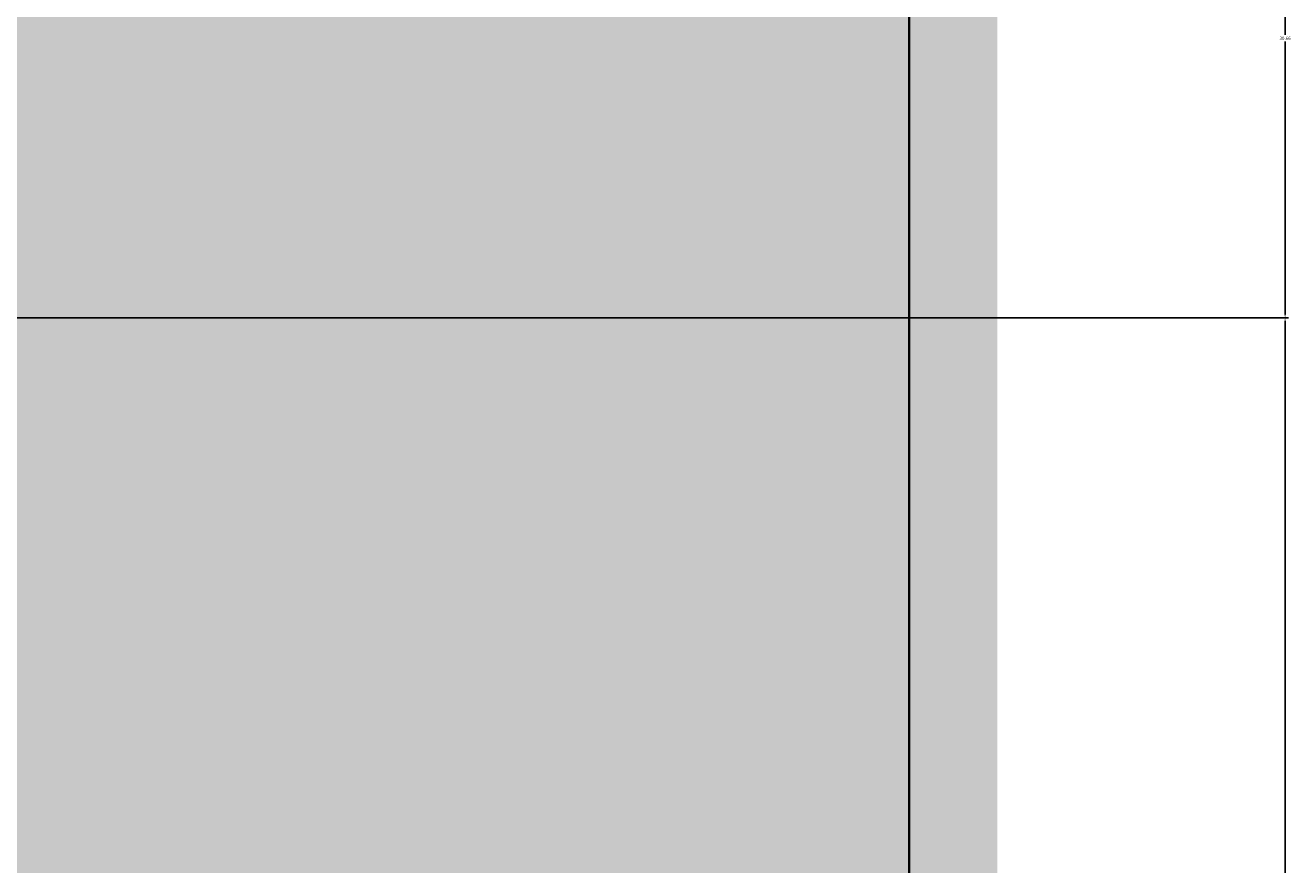
# Model space of a CAD drawing. Units: feet. Extents: x 2695 to 2912, y 795 to 1139.
# Tile 31 of 83: x 2842 to 2912, y 845 to 891. Entities that reach past the tile are written whole.
import ezdxf

# ---------------------------------------------------------------- set-up
doc = ezdxf.new("R2010")
doc.units = ezdxf.units.FT
for name, color, linetype, lineweight in [('A-ANNO-DIMS', 2, 'Continuous', 18), ('A-ELEV', 7, 'Continuous', 35), ('A-ELEV-PATT', 252, 'Continuous', 13)]:
    doc.layers.add(name, color=color, linetype=linetype, lineweight=lineweight)
doc.styles.get("Standard").update_dxf_attribs({"font": 'arial.ttf'})
doc.dimstyles.get("Standard").update_dxf_attribs({"dimtxt": 0.18, "dimasz": 0.18, "dimexe": 0.18, "dimexo": 0.0625, "dimgap": 0.09, "dimtad": 0, "dimtih": 1, "dimtoh": 1, "dimdec": 1, "dimzin": 0, "dimdsep": 46, "dimlunit": 3, "dimtxsty": 'Standard', "dimcen": 0.09, "dimadec": 0, "dimazin": 0, "dimtfac": 1, "dimtdec": 1, "dimtofl": 0, "dimtmove": 0, "dimatfit": 3, "dimfxl": 1, "dimtolj": 1, "dimtzin": 0, "dimarcsym": 0})

# ---------------------------------------------------------------- blocks, each defined once
blk = doc.blocks.new('*D13')
at = {"layer": 'A-ANNO-DIMS', "color": 0, "lineweight": -2, "transparency": 16777216}
for p, q in [((2758.214, 874.857), (2911.424, 874.857)), ((2911.244, 874.677), (2911.244, 843.076)), ((2911.244, 811.111), (2911.244, 842.712)), ((2890.699, 810.931), (2911.424, 810.931))]:
    blk.add_line(p, q, dxfattribs=at)
at = {"layer": 'A-ANNO-DIMS', "color": 0, "transparency": 16777216}
for points in [[(2911.214, 874.677), (2911.274, 874.677), (2911.244, 874.857)], [(2911.214, 811.111), (2911.274, 811.111), (2911.244, 810.931)]]:
    blk.add_solid(points, dxfattribs=at)
at = {"layer": 'Defpoints', "color": 0, "transparency": 16777216}
for p in [(2758.151, 874.857), (2911.244, 874.857), (2890.636, 810.931)]:
    blk.add_point(p, dxfattribs=at)
at = {"layer": 'A-ANNO-DIMS', "color": 0, "transparency": 16777216, "insert": (2911.244, 842.894), "char_height": 0.18, "attachment_point": 5}
blk.add_mtext('\\A1;63.93', dxfattribs=at)
blk = doc.blocks.new('*D14')
at = {"layer": 'A-ANNO-DIMS', "color": 0, "lineweight": -2, "transparency": 16777216}
for p, q in [((2838.439, 905.514), (2911.424, 905.514)), ((2911.244, 905.334), (2911.244, 890.368)), ((2911.244, 875.037), (2911.244, 890.004)), ((2758.214, 874.857), (2911.424, 874.857))]:
    blk.add_line(p, q, dxfattribs=at)
at = {"layer": 'A-ANNO-DIMS', "color": 0, "transparency": 16777216}
for points in [[(2911.214, 905.334), (2911.274, 905.334), (2911.244, 905.514)], [(2911.214, 875.037), (2911.274, 875.037), (2911.244, 874.857)]]:
    blk.add_solid(points, dxfattribs=at)
at = {"layer": 'Defpoints', "color": 0, "transparency": 16777216}
for p in [(2838.377, 905.514), (2911.244, 905.514), (2758.151, 874.857)]:
    blk.add_point(p, dxfattribs=at)
at = {"layer": 'A-ANNO-DIMS', "color": 0, "transparency": 16777216, "insert": (2911.244, 890.186), "char_height": 0.18, "attachment_point": 5}
blk.add_mtext('\\A1;30.66', dxfattribs=at)

msp = doc.modelspace()

# ---------------------------------------------------------------- hatches: boundary and pattern name
at = {"layer": 'A-ELEV-PATT'}
h = msp.add_hatch(color=256, dxfattribs=at)
h.set_gradient(color1=(147, 149, 152), color2=(147, 149, 152), tint=1)
h.paths.add_polyline_path([(2770.6361, 1118.4096), (2710.6361, 1118.4096), (2710.6361, 1062.9306), (2770.6361, 1062.9306)])
h.paths.add_polyline_path([(2890.6361, 1103.3378), (2770.6361, 1103.3378), (2770.6361, 1062.9306), (2890.6361, 1062.9306)])
h.paths.add_polyline_path([(2730.7081, 1048.1052), (2755.1125, 1048.1052), (2755.1125, 936.9306), (2770.6361, 936.9306), (2770.6361, 1050.3105), (2715.8852, 1050.3105), (2715.8852, 936.9306), (2730.7081, 936.9306)])
h.paths.add_polyline_path([(2890.6361, 1050.3105), (2770.6361, 1050.3105), (2770.6361, 971.9673), (2778.0341, 971.9673), (2778.0341, 1020.8235), (2843.575, 1020.8235), (2843.575, 971.9673), (2890.6361, 971.9673)])
h.paths.add_polyline_path([(2888.1882, 970.7156), (2843.575, 970.7156), (2843.575, 964.8267), (2888.1882, 964.8267)])
h.paths.add_polyline_path([(2888.1882, 964.1328), (2843.575, 964.1328), (2843.575, 956.614), (2888.1882, 956.614)])
h.paths.add_polyline_path([(2888.1882, 955.9202), (2843.575, 955.9202), (2843.575, 949.2892), (2888.1882, 949.2892)])
h.paths.add_polyline_path([(2888.1882, 948.5954), (2843.575, 948.5954), (2843.575, 941.3507), (2888.1882, 941.3507)])
h.paths.add_polyline_path([(2888.1882, 940.6569), (2843.575, 940.6569), (2843.575, 936.9306), (2888.1882, 936.9306)])
h.paths.add_polyline_path([(2890.6361, 970.7156), (2888.9368, 970.7156), (2888.9368, 964.8267), (2890.6361, 964.8267)])
h.paths.add_polyline_path([(2890.6361, 964.1328), (2888.9368, 964.1328), (2888.9368, 956.614), (2890.6361, 956.614)])
h.paths.add_polyline_path([(2890.6361, 955.9202), (2888.9368, 955.9202), (2888.9368, 949.2892), (2890.6361, 949.2892)])
h.paths.add_polyline_path([(2890.6361, 940.6569), (2888.9368, 940.6569), (2888.9368, 936.9306), (2890.6361, 936.9306)])
h.paths.add_polyline_path([(2890.6361, 948.5954), (2888.9368, 948.5954), (2888.9368, 941.3507), (2890.6361, 941.3507)])
h.paths.add_polyline_path([(2772.5216, 970.7156), (2770.6361, 970.7156), (2770.6361, 964.8267), (2772.5216, 964.8267)])
h.paths.add_polyline_path([(2772.5216, 964.1328), (2770.6361, 964.1328), (2770.6361, 956.614), (2772.5216, 956.614)])
h.paths.add_polyline_path([(2772.5216, 955.9202), (2770.6361, 955.9202), (2770.6361, 949.2892), (2772.5216, 949.2892)])
h.paths.add_polyline_path([(2772.5216, 948.5954), (2770.6361, 948.5954), (2770.6361, 941.3507), (2772.5216, 941.3507)])
h.paths.add_polyline_path([(2772.5216, 940.6569), (2770.6361, 940.6569), (2770.6361, 936.9306), (2772.5216, 936.9306)])
h.paths.add_polyline_path([(2778.0341, 940.6569), (2773.2702, 940.6569), (2773.2702, 936.9306), (2778.0341, 936.9306)])
h.paths.add_polyline_path([(2778.0341, 970.7156), (2773.2702, 970.7156), (2773.2702, 964.8267), (2778.0341, 964.8267)])
h.paths.add_polyline_path([(2778.0341, 964.1328), (2773.2702, 964.1328), (2773.2702, 956.614), (2778.0341, 956.614)])
h.paths.add_polyline_path([(2778.0341, 955.9202), (2773.2702, 955.9202), (2773.2702, 949.2892), (2778.0341, 949.2892)])
h.paths.add_polyline_path([(2778.0341, 948.5954), (2773.2702, 948.5954), (2773.2702, 941.3507), (2778.0341, 941.3507)])
h.paths.add_polyline_path([(2810.0407, 940.6569), (2780.0341, 940.6569), (2780.0341, 936.9306), (2810.0407, 936.9306)])
h.paths.add_polyline_path([(2890.6361, 924.3105), (2770.6361, 924.3105), (2770.6361, 810.9306), (2773.5029, 810.9306), (2773.5029, 905.5143), (2805.9398, 905.5143), (2838.3767, 905.5143), (2838.3767, 810.9306), (2890.6361, 810.9306)])
h = msp.add_hatch(color=256, dxfattribs=at)
h.set_gradient(color1=(255, 255, 255), tint=1)
h.paths.add_polyline_path([(2895.4694, 1107.8588), (2890.6361, 1107.8588), (2890.6361, 810.9306), (2895.4694, 810.9306)])

# ---------------------------------------------------------------- linework, layer by layer
at = {"layer": 'A-ELEV'}
for p, q in [((2890.6361, 810.9306), (2890.6361, 1107.8588)), ((2890.6361, 1062.9306), (2890.6361, 810.9306))]:
    msp.add_line(p, q, dxfattribs=at)

# ---------------------------------------------------------------- dimensions: what is measured, and where the dimension line sits
at = {"layer": 'A-ANNO-DIMS'}
for base, p1, p2, picture, middle in [((2911.2444, 905.5143), (2758.1515, 874.8571), (2838.3767, 905.5143), '*D14', (2911.2444, 890.1857)), ((2911.2444, 874.8571), (2890.6361, 810.9306), (2758.1515, 874.8571), '*D13', (2911.2444, 842.8938))]:
    dim = msp.add_linear_dim(base=base, p1=p1, p2=p2, angle=90, dimstyle='Standard', override={"dimdec": 2, "dimlfac": 1, "dimrnd": 0, "dimzin": 0, "dimdsep": 46, "dimlunit": 2}, dxfattribs=at)
    dim.commit()
    dim.dimension.update_dxf_attribs({"geometry": picture, "text_midpoint": middle})

doc.saveas('drawing.dxf')
